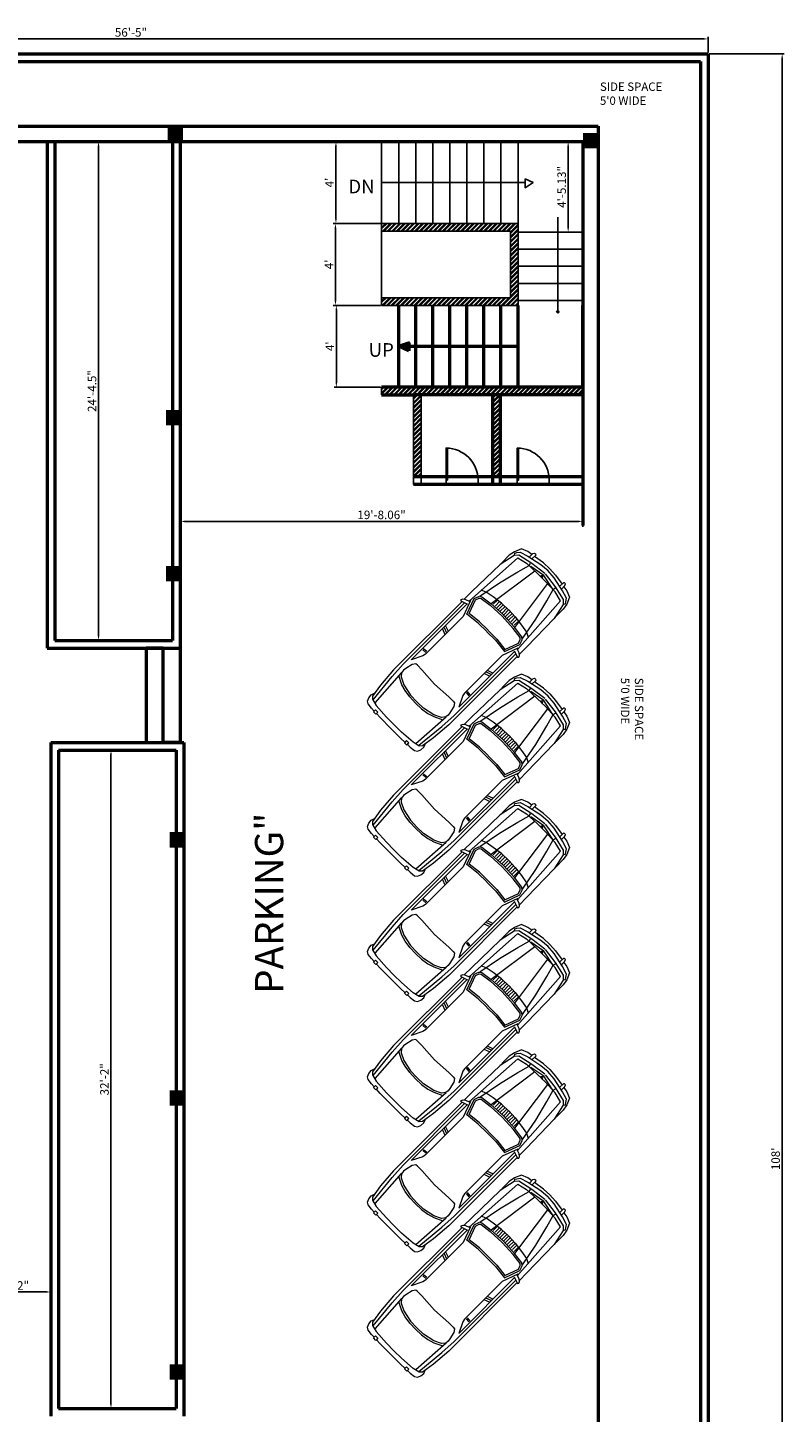
# Model space of a CAD drawing. Units: inches. Extents: x -2733 to 3435, y -338 to 1843.
# Tile 4 of 7: x -2146 to -1702, y 764 to 1575. Entities that reach past the tile are written whole.
import ezdxf

# ---------------------------------------------------------------- set-up
doc = ezdxf.new("R2010")
doc.units = ezdxf.units.IN
doc.header["$PDMODE"] = 34
for name, color, linetype, lineweight in [('A-ANNO-DIMS', 2, 'Continuous', 18), ('A-ANNO-TEXT', 7, 'Continuous', 18), ('A-AREA-IDEN', 3, 'Continuous', 18), ('A-COLS', 1, 'Continuous', 35), ('A-DOOR', 1, 'Continuous', 25), ('A-FLOR-STRS', 4, 'Continuous', 25), ('A-WALL', 7, 'Continuous', 50), ('A-WALL-PATT', 8, 'Continuous', 13), ('C-PRKG', 8, 'Continuous', 18)]:
    doc.layers.add(name, color=color, linetype=linetype, lineweight=lineweight)
doc.styles.get("Standard").update_dxf_attribs({"font": 'arial.ttf'})
doc.styles.add('YQ_DIM', font='SUPEROS.SHX', dxfattribs={"width": 0.8, "bigfont": 'HZDX.SHX'})
doc.dimstyles.new('ISO-25', dxfattribs={"dimtxt": 5, "dimasz": 2.5, "dimexe": 1.25, "dimexo": 0.625, "dimtad": 1, "dimlunit": 3, "dimtxsty": 'Standard', "dimcen": 2.5, "dimadec": 0, "dimazin": 0, "dimtfac": 1, "dimtmove": 0, "dimatfit": 3, "dimfxl": 1, "dimarcsym": 0})

# ---------------------------------------------------------------- blocks, each defined once
blk = doc.blocks.new('A$C49703025')
for p, q in [((-0.089, 0.573), (-0.077, 0.686)), ((-0.077, 0.686), (-0.044, 0.735)), ((-0.044, 0.735), (0.024, 0.765)), ((0.057, 0.691), (0.02, 0.543)), ((0.024, 0.765), (0.105, 0.775)), ((0.881, 0.661), (0.04, 0.607)), ((0.105, 0.735), (0.057, 0.691)), ((0.061, 0.671), (0.683, 0.735)), ((0.388, 0.78), (0.105, 0.735)), ((0.105, 0.775), (0.174, 0.75)), ((0.804, 0.813), (0.388, 0.78)), ((0.683, 0.735), (1.027, 0.755)), ((0.707, 0.469), (0.792, 0.652)), ((0.808, 0.597), (0.732, 0.444)), ((2.822, 0.813), (0.804, 0.813)), ((0.877, 0.652), (0.808, 0.597)), ((0.942, 0.661), (0.877, 0.652)), ((1.002, 0.652), (0.942, 0.661)), ((1.152, 0.617), (1.002, 0.652)), ((1.027, 0.755), (2.841, 0.755)), ((1.217, 0.573), (1.152, 0.617)), ((1.443, 0.586), (1.212, 0.702)), ((1.212, 0.702), (2.85, 0.702)), ((1.507, 0.575), (1.443, 0.586)), ((1.538, 0.592), (1.529, 0.68)), ((1.566, 0.592), (1.557, 0.68)), ((2.125, 0.696), (2.083, 0.58)), ((2.174, 0.695), (2.132, 0.579)), ((2.219, 0.697), (2.178, 0.581)), ((2.958, 0.702), (2.618, 0.575)), ((2.707, 0.554), (3.041, 0.676)), ((2.747, 0.529), (3.041, 0.637)), ((2.816, 0.829), (2.838, 0.849)), ((2.864, 0.684), (2.816, 0.829)), ((2.838, 0.849), (2.874, 0.835)), ((2.874, 0.835), (2.905, 0.791)), ((3.1, 0.813), (2.89, 0.813)), ((2.905, 0.791), (2.932, 0.714)), ((2.932, 0.714), (4.286, 0.632)), ((3.041, 0.676), (3.144, 0.639)), ((3.041, 0.637), (3.122, 0.608)), ((3.929, 0.795), (3.1, 0.813)), ((3.122, 0.608), (3.148, 0.576)), ((3.144, 0.639), (3.183, 0.591)), ((3.163, 0.627), (3.648, 0.536)), ((3.183, 0.591), (3.217, 0.343)), ((3.317, 0.591), (3.271, 0.695)), ((3.35, 0.417), (3.317, 0.591)), ((4.269, 0.722), (3.929, 0.795)), ((3.993, 0.795), (3.965, 0.787)), ((4.2, 0.795), (3.993, 0.795)), ((4.328, 0.77), (4.2, 0.795)), ((4.343, 0.656), (4.269, 0.722)), ((4.279, 0.724), (4.312, 0.747)), ((4.286, 0.632), (4.337, 0.422)), ((4.312, 0.747), (4.35, 0.724)), ((4.472, 0.711), (4.328, 0.77)), ((4.412, 0.343), (4.343, 0.656)), ((4.35, 0.724), (4.407, 0.681)), ((4.407, 0.681), (4.461, 0.513)), ((4.525, 0.578), (4.472, 0.711)), ((-0.113, 0.489), (-0.053, 0.489)), ((-0.113, 0.42), (-0.113, 0.489)), ((-0.053, 0.42), (-0.113, 0.42)), ((-0.101, 0.306), (-0.096, 0.42)), ((-0.101, 0), (-0.101, 0.306)), ((-0.093, 0.489), (-0.089, 0.573)), ((-0.053, 0.489), (-0.053, 0.42)), ((0.02, 0.543), (0, 0.222)), ((0.643, 0.173), (0.667, 0.336)), ((0.667, 0.336), (0.707, 0.469)), ((0.732, 0.444), (0.679, 0.193)), ((1.196, 0), (1.221, 0.4)), ((1.221, 0.528), (1.217, 0.573)), ((1.221, 0.4), (1.221, 0.528)), ((2.618, 0.575), (1.507, 0.575)), ((2.741, 0.254), (2.707, 0.554)), ((2.778, 0.256), (2.747, 0.529)), ((3.148, 0.576), (3.18, 0.34)), ((3.18, 0.34), (3.198, 0)), ((3.217, 0.343), (3.235, 0.002)), ((3.22, 0.35), (4.35, 0.19)), ((3.241, 0.309), (3.365, 0.309)), ((3.38, 0.202), (3.35, 0.417)), ((3.648, 0.536), (4.083, 0.427)), ((4.083, 0.427), (4.344, 0.354)), ((4.337, 0.422), (4.348, 0.111)), ((4.344, 0.354), (4.395, 0.364)), ((4.415, -0.011), (4.354, 0.313)), ((4.395, 0.364), (4.404, 0.379)), ((4.456, 0.006), (4.412, 0.343)), ((4.461, 0.513), (4.529, 0.197)), ((4.473, 0.474), (4.574, 0.474)), ((4.592, 0.408), (4.49, 0.408)), ((4.542, 0.474), (4.525, 0.578)), ((4.59, 0.18), (4.553, 0.408)), ((4.574, 0.474), (4.606, 0.455)), ((4.609, 0.429), (4.592, 0.408)), ((4.606, 0.455), (4.609, 0.429)), ((-0.101, 0), (-0.101, -0.306)), ((0, 0.222), (0, 0)), ((0, -0.222), (0, 0)), ((0.635, 0), (0.643, 0.173)), ((0.635, 0), (0.643, -0.173)), ((0.679, 0.193), (0.671, 0)), ((0.679, -0.193), (0.671, 0)), ((1.196, 0), (1.221, -0.4)), ((2.744, 0.002), (2.741, 0.254)), ((2.781, 0.003), (2.778, 0.256)), ((3.241, 0.257), (3.373, 0.257)), ((3.241, 0.206), (3.382, 0.206)), ((3.241, 0.154), (3.382, 0.154)), ((3.241, 0.103), (3.382, 0.103)), ((3.241, 0.051), (3.382, 0.051)), ((3.241, 0), (3.382, 0)), ((3.386, 0.002), (3.38, 0.202)), ((4.348, 0.111), (4.348, -0.004)), ((4.348, -0.111), (4.348, 0.004)), ((4.363, 0.028), (4.359, 0.005)), ((4.359, 0.005), (4.363, -0.023)), ((4.386, 0.005), (4.363, 0.028)), ((4.529, 0.197), (4.546, -0.002)), ((4.529, -0.197), (4.546, 0.002)), ((4.599, 0), (4.59, 0.18)), ((4.599, 0), (4.59, -0.18)), ((0.02, -0.543), (0, -0.222)), ((0.643, -0.173), (0.667, -0.336)), ((0.732, -0.444), (0.679, -0.193)), ((2.741, -0.254), (2.707, -0.554)), ((2.744, -0.002), (2.741, -0.254)), ((2.778, -0.256), (2.747, -0.529)), ((2.781, -0.003), (2.778, -0.256)), ((3.18, -0.34), (3.198, 0)), ((3.217, -0.343), (3.235, -0.002)), ((3.22, -0.35), (4.35, -0.19)), ((3.241, -0.051), (3.382, -0.051)), ((3.241, -0.103), (3.382, -0.103)), ((3.241, -0.154), (3.382, -0.154)), ((3.241, -0.206), (3.382, -0.206)), ((3.241, -0.257), (3.373, -0.257)), ((3.38, -0.202), (3.35, -0.417)), ((3.386, -0.002), (3.38, -0.202)), ((4.337, -0.422), (4.348, -0.111)), ((4.344, -0.347), (4.415, -0.011)), ((4.401, 0), (4.354, 0)), ((4.363, -0.023), (4.382, -0.011)), ((4.456, -0.006), (4.412, -0.343)), ((4.461, -0.513), (4.529, -0.197)), ((4.59, -0.18), (4.553, -0.408)), ((-0.053, -0.42), (-0.113, -0.42)), ((-0.113, -0.42), (-0.113, -0.489)), ((-0.113, -0.489), (-0.053, -0.489)), ((-0.101, -0.306), (-0.096, -0.42)), ((-0.093, -0.489), (-0.089, -0.573)), ((-0.089, -0.573), (-0.077, -0.686)), ((-0.053, -0.489), (-0.053, -0.42)), ((0.057, -0.691), (0.02, -0.543)), ((0.667, -0.336), (0.707, -0.469)), ((0.707, -0.469), (0.792, -0.652)), ((0.808, -0.597), (0.732, -0.444)), ((1.217, -0.573), (1.152, -0.617)), ((1.221, -0.528), (1.217, -0.573)), ((1.221, -0.4), (1.221, -0.528)), ((1.507, -0.575), (1.443, -0.586)), ((2.618, -0.575), (1.507, -0.575)), ((2.958, -0.702), (2.618, -0.575)), ((2.707, -0.554), (3.041, -0.676)), ((2.747, -0.529), (3.041, -0.637)), ((3.122, -0.608), (3.148, -0.576)), ((3.148, -0.576), (3.18, -0.34)), ((3.163, -0.627), (3.648, -0.536)), ((3.183, -0.591), (3.217, -0.343)), ((3.241, -0.309), (3.365, -0.309)), ((3.35, -0.417), (3.317, -0.591)), ((3.648, -0.536), (4.083, -0.427)), ((4.083, -0.427), (4.344, -0.354)), ((4.286, -0.632), (4.337, -0.422)), ((4.412, -0.343), (4.343, -0.656)), ((4.344, -0.354), (4.395, -0.364)), ((4.395, -0.364), (4.404, -0.379)), ((4.407, -0.681), (4.461, -0.513)), ((4.525, -0.578), (4.472, -0.711)), ((4.473, -0.474), (4.574, -0.474)), ((4.592, -0.408), (4.49, -0.408)), ((4.542, -0.474), (4.525, -0.578)), ((4.574, -0.474), (4.606, -0.455)), ((4.609, -0.429), (4.592, -0.408)), ((4.606, -0.455), (4.609, -0.429)), ((-0.077, -0.686), (-0.044, -0.735)), ((-0.044, -0.735), (0.024, -0.765)), ((0.024, -0.765), (0.105, -0.775)), ((0.881, -0.661), (0.04, -0.607)), ((0.105, -0.735), (0.057, -0.691)), ((0.061, -0.671), (0.683, -0.735)), ((0.388, -0.78), (0.105, -0.735)), ((0.105, -0.775), (0.174, -0.75)), ((0.804, -0.813), (0.388, -0.78)), ((0.683, -0.735), (1.027, -0.755)), ((2.822, -0.813), (0.804, -0.813)), ((0.877, -0.652), (0.808, -0.597)), ((0.942, -0.661), (0.877, -0.652)), ((1.002, -0.652), (0.942, -0.661)), ((1.152, -0.617), (1.002, -0.652)), ((1.027, -0.755), (2.841, -0.755)), ((1.443, -0.586), (1.212, -0.702)), ((1.212, -0.702), (2.85, -0.702)), ((1.538, -0.592), (1.529, -0.68)), ((1.566, -0.592), (1.557, -0.68)), ((2.125, -0.696), (2.083, -0.58)), ((2.174, -0.695), (2.132, -0.579)), ((2.219, -0.697), (2.178, -0.581)), ((2.864, -0.684), (2.816, -0.829)), ((2.816, -0.829), (2.838, -0.849)), ((2.838, -0.849), (2.874, -0.835)), ((2.874, -0.835), (2.905, -0.791)), ((3.1, -0.813), (2.89, -0.813)), ((2.905, -0.791), (2.932, -0.714)), ((2.932, -0.714), (4.286, -0.632)), ((3.041, -0.637), (3.122, -0.608)), ((3.041, -0.676), (3.144, -0.639)), ((3.929, -0.795), (3.1, -0.813)), ((3.144, -0.639), (3.183, -0.591)), ((3.317, -0.591), (3.271, -0.695)), ((4.269, -0.722), (3.929, -0.795)), ((3.993, -0.795), (3.965, -0.787)), ((4.2, -0.795), (3.993, -0.795)), ((4.328, -0.77), (4.2, -0.795)), ((4.343, -0.656), (4.269, -0.722)), ((4.279, -0.724), (4.312, -0.747)), ((4.312, -0.747), (4.35, -0.724)), ((4.472, -0.711), (4.328, -0.77)), ((4.35, -0.724), (4.407, -0.681))]:
    blk.add_line(p, q)
blk = doc.blocks.new('*D6')
at = {"layer": 'A-ANNO-DIMS', "color": 0, "lineweight": -2, "transparency": 16777216}
for p, q in [((-1745.94, 1560.13), (-1701.93, 1560.13)), ((-1703.18, 1557.63), (-1703.18, 266.63)), ((-1745.94, 264.13), (-1701.93, 264.13))]:
    blk.add_line(p, q, dxfattribs=at)
at = {"layer": 'A-ANNO-DIMS', "color": 0, "lineweight": 20, "transparency": 16777216}
for points in [[(-1703.6, 1557.63), (-1702.76, 1557.63), (-1703.18, 1560.13)], [(-1703.6, 266.63), (-1702.76, 266.63), (-1703.18, 264.13)]]:
    blk.add_solid(points, dxfattribs=at)
at = {"layer": 'Defpoints', "color": 0, "lineweight": 20, "transparency": 16777216}
for p in [(-1746.57, 1560.13), (-1746.57, 264.13), (-1703.18, 264.13)]:
    blk.add_point(p, dxfattribs=at)
at = {"layer": 'A-ANNO-DIMS', "color": 0, "transparency": 16777216, "insert": (-1706.36, 912.13), "char_height": 5, "attachment_point": 5, "rotation": 90}
blk.add_mtext("108'", dxfattribs=at)
blk = doc.blocks.new('*D8')
at = {"layer": 'A-ANNO-DIMS', "color": 0, "lineweight": -2, "transparency": 16777216}
for p, q in [((-2093.63, 1151.77), (-2098.01, 1151.77)), ((-2096.76, 1149.27), (-2096.76, 768.27)), ((-2093.63, 765.77), (-2098.01, 765.77))]:
    blk.add_line(p, q, dxfattribs=at)
at = {"layer": 'A-ANNO-DIMS', "color": 0, "lineweight": 20, "transparency": 16777216}
for points in [[(-2097.18, 1149.27), (-2096.34, 1149.27), (-2096.76, 1151.77)], [(-2097.18, 768.27), (-2096.34, 768.27), (-2096.76, 765.77)]]:
    blk.add_solid(points, dxfattribs=at)
at = {"layer": 'Defpoints', "color": 0, "lineweight": 20, "transparency": 16777216}
for p in [(-2093.01, 1151.77), (-2096.76, 765.77), (-2093.01, 765.77)]:
    blk.add_point(p, dxfattribs=at)
at = {"layer": 'A-ANNO-DIMS', "color": 0, "transparency": 16777216, "insert": (-2099.94, 958.77), "char_height": 5, "attachment_point": 5, "rotation": 90}
blk.add_mtext('32\'-2"', dxfattribs=at)
blk = doc.blocks.new('*D9')
at = {"layer": 'A-ANNO-DIMS', "color": 0, "lineweight": -2, "transparency": 16777216}
for p, q in [((-2182.13, 829.34), (-2182.13, 835.34)), ((-2179.63, 834.09), (-2134.51, 834.09)), ((-2132.01, 829.34), (-2132.01, 835.34))]:
    blk.add_line(p, q, dxfattribs=at)
at = {"layer": 'A-ANNO-DIMS', "color": 0, "lineweight": 20, "transparency": 16777216}
for points in [[(-2179.63, 834.5), (-2179.63, 833.67), (-2182.13, 834.09)], [(-2134.51, 834.5), (-2134.51, 833.67), (-2132.01, 834.09)]]:
    blk.add_solid(points, dxfattribs=at)
at = {"layer": 'Defpoints', "color": 0, "lineweight": 20, "transparency": 16777216}
for p in [(-2182.13, 828.71), (-2132.01, 834.09), (-2132.01, 828.71)]:
    blk.add_point(p, dxfattribs=at)
at = {"layer": 'A-ANNO-DIMS', "color": 0, "transparency": 16777216, "insert": (-2157.07, 837.22), "char_height": 5, "attachment_point": 5}
blk.add_mtext('4\'-2.12"', dxfattribs=at)
blk = doc.blocks.new('*D12')
at = {"layer": 'A-ANNO-DIMS', "color": 0, "lineweight": -2, "transparency": 16777216}
for p, q in [((-2094.22, 1508.58), (-2105.31, 1508.58)), ((-2104.06, 1506.08), (-2104.06, 1218.58)), ((-2100.09, 1216.08), (-2105.31, 1216.08))]:
    blk.add_line(p, q, dxfattribs=at)
at = {"layer": 'A-ANNO-DIMS', "color": 0, "lineweight": 20, "transparency": 16777216}
for points in [[(-2104.47, 1506.08), (-2103.64, 1506.08), (-2104.06, 1508.58)], [(-2104.47, 1218.58), (-2103.64, 1218.58), (-2104.06, 1216.08)]]:
    blk.add_solid(points, dxfattribs=at)
at = {"layer": 'Defpoints', "color": 0, "lineweight": 20, "transparency": 16777216}
for p in [(-2093.59, 1508.58), (-2104.06, 1216.08), (-2099.46, 1216.08)]:
    blk.add_point(p, dxfattribs=at)
at = {"layer": 'A-ANNO-DIMS', "color": 0, "transparency": 16777216, "insert": (-2107.23, 1362.33), "char_height": 5, "attachment_point": 5, "rotation": 90}
blk.add_mtext('24\'-4.5"', dxfattribs=at)
blk = doc.blocks.new('*D13')
at = {"layer": 'A-ANNO-DIMS', "color": 0, "lineweight": -2, "transparency": 16777216}
for p, q in [((-2423.57, 1560.75), (-2423.57, 1570.04)), ((-2421.07, 1568.79), (-1749.07, 1568.79)), ((-1746.57, 1560.75), (-1746.57, 1570.04))]:
    blk.add_line(p, q, dxfattribs=at)
at = {"layer": 'A-ANNO-DIMS', "color": 0, "lineweight": 20, "transparency": 16777216}
for points in [[(-2421.07, 1569.21), (-2421.07, 1568.38), (-2423.57, 1568.79)], [(-1749.07, 1569.21), (-1749.07, 1568.38), (-1746.57, 1568.79)]]:
    blk.add_solid(points, dxfattribs=at)
at = {"layer": 'Defpoints', "color": 0, "lineweight": 20, "transparency": 16777216}
for p in [(-1746.57, 1568.79), (-2423.57, 1560.13), (-1746.57, 1560.13)]:
    blk.add_point(p, dxfattribs=at)
at = {"layer": 'A-ANNO-DIMS', "color": 0, "transparency": 16777216, "insert": (-2085.07, 1571.97), "char_height": 5, "attachment_point": 5}
blk.add_mtext('56\'-5"', dxfattribs=at)
blk = doc.blocks.new('*D14')
at = {"layer": 'A-ANNO-DIMS', "color": 0, "lineweight": -2, "transparency": 16777216}
for p, q in [((-1830.95, 1508.58), (-1827.42, 1508.58)), ((-1828.67, 1506.08), (-1828.67, 1457.96)), ((-1828.59, 1455.46), (-1827.42, 1455.46))]:
    blk.add_line(p, q, dxfattribs=at)
at = {"layer": 'A-ANNO-DIMS', "color": 0, "lineweight": 20, "transparency": 16777216}
for points in [[(-1829.09, 1506.08), (-1828.26, 1506.08), (-1828.67, 1508.58)], [(-1829.09, 1457.96), (-1828.26, 1457.96), (-1828.67, 1455.46)]]:
    blk.add_solid(points, dxfattribs=at)
at = {"layer": 'Defpoints', "color": 0, "lineweight": 20, "transparency": 16777216}
for p in [(-1831.58, 1508.58), (-1829.22, 1455.46), (-1828.67, 1455.46)]:
    blk.add_point(p, dxfattribs=at)
at = {"layer": 'A-ANNO-DIMS', "color": 0, "transparency": 16777216, "insert": (-1831.85, 1482.02), "char_height": 5, "attachment_point": 5, "rotation": 90}
blk.add_mtext('4\'-5.13"', dxfattribs=at)
blk = doc.blocks.new('*D15')
at = {"layer": 'A-ANNO-DIMS', "color": 0, "lineweight": -2, "transparency": 16777216}
for p, q in [((-1963.16, 1508.58), (-1966.11, 1508.58)), ((-1964.86, 1506.08), (-1964.86, 1463.08)), ((-1938.69, 1460.58), (-1966.11, 1460.58))]:
    blk.add_line(p, q, dxfattribs=at)
at = {"layer": 'A-ANNO-DIMS', "color": 0, "lineweight": 20, "transparency": 16777216}
for points in [[(-1965.27, 1506.08), (-1964.44, 1506.08), (-1964.86, 1508.58)], [(-1965.27, 1463.08), (-1964.44, 1463.08), (-1964.86, 1460.58)]]:
    blk.add_solid(points, dxfattribs=at)
at = {"layer": 'Defpoints', "color": 0, "lineweight": 20, "transparency": 16777216}
for p in [(-1962.53, 1508.58), (-1964.86, 1460.58), (-1938.07, 1460.58)]:
    blk.add_point(p, dxfattribs=at)
at = {"layer": 'A-ANNO-DIMS', "color": 0, "transparency": 16777216, "insert": (-1967.98, 1484.58), "char_height": 5, "attachment_point": 5, "rotation": 90}
blk.add_mtext("4'", dxfattribs=at)
blk = doc.blocks.new('*D16')
at = {"layer": 'A-ANNO-DIMS', "color": 0, "lineweight": -2, "transparency": 16777216}
for p, q in [((-1938.69, 1460.58), (-1966.4, 1460.58)), ((-1965.15, 1458.08), (-1965.15, 1415.08)), ((-1938.69, 1412.58), (-1966.4, 1412.58))]:
    blk.add_line(p, q, dxfattribs=at)
at = {"layer": 'A-ANNO-DIMS', "color": 0, "lineweight": 20, "transparency": 16777216}
for points in [[(-1965.56, 1458.08), (-1964.73, 1458.08), (-1965.15, 1460.58)], [(-1965.56, 1415.08), (-1964.73, 1415.08), (-1965.15, 1412.58)]]:
    blk.add_solid(points, dxfattribs=at)
at = {"layer": 'Defpoints', "color": 0, "lineweight": 20, "transparency": 16777216}
for p in [(-1938.07, 1460.58), (-1965.15, 1412.58), (-1938.07, 1412.58)]:
    blk.add_point(p, dxfattribs=at)
at = {"layer": 'A-ANNO-DIMS', "color": 0, "transparency": 16777216, "insert": (-1968.27, 1436.58), "char_height": 5, "attachment_point": 5, "rotation": 90}
blk.add_mtext("4'", dxfattribs=at)
blk = doc.blocks.new('*D17')
at = {"layer": 'A-ANNO-DIMS', "color": 0, "lineweight": -2, "transparency": 16777216}
for p, q in [((-1938.69, 1412.58), (-1965.87, 1412.58)), ((-1964.62, 1410.08), (-1964.62, 1367.08)), ((-1938.69, 1364.58), (-1965.87, 1364.58))]:
    blk.add_line(p, q, dxfattribs=at)
at = {"layer": 'A-ANNO-DIMS', "color": 0, "lineweight": 20, "transparency": 16777216}
for points in [[(-1965.04, 1410.08), (-1964.21, 1410.08), (-1964.62, 1412.58)], [(-1965.04, 1367.08), (-1964.21, 1367.08), (-1964.62, 1364.58)]]:
    blk.add_solid(points, dxfattribs=at)
at = {"layer": 'Defpoints', "color": 0, "lineweight": 20, "transparency": 16777216}
for p in [(-1938.07, 1412.58), (-1964.62, 1364.58), (-1938.07, 1364.58)]:
    blk.add_point(p, dxfattribs=at)
at = {"layer": 'A-ANNO-DIMS', "color": 0, "transparency": 16777216, "insert": (-1967.75, 1388.58), "char_height": 5, "attachment_point": 5, "rotation": 90}
blk.add_mtext("4'", dxfattribs=at)
blk = doc.blocks.new('*D18')
at = {"layer": 'A-ANNO-DIMS', "color": 0, "lineweight": -2, "transparency": 16777216}
for p, q in [((-2056.13, 1282.79), (-2056.13, 1287.15)), ((-2053.63, 1285.9), (-1822.57, 1285.9)), ((-1820.07, 1282.79), (-1820.07, 1287.15))]:
    blk.add_line(p, q, dxfattribs=at)
at = {"layer": 'A-ANNO-DIMS', "color": 0, "lineweight": 20, "transparency": 16777216}
for points in [[(-2053.63, 1286.32), (-2053.63, 1285.49), (-2056.13, 1285.9)], [(-1822.57, 1286.32), (-1822.57, 1285.49), (-1820.07, 1285.9)]]:
    blk.add_solid(points, dxfattribs=at)
at = {"layer": 'Defpoints', "color": 0, "lineweight": 20, "transparency": 16777216}
for p in [(-1820.07, 1285.9), (-2056.13, 1282.16), (-1820.07, 1282.16)]:
    blk.add_point(p, dxfattribs=at)
at = {"layer": 'A-ANNO-DIMS', "color": 0, "transparency": 16777216, "insert": (-1938.1, 1289.08), "char_height": 5, "width": 26.4154, "attachment_point": 5}
blk.add_mtext('19\'-8.06"', dxfattribs=at)
blk = doc.blocks.new('*U21')
for p, q in [((0, 0), (0, -6)), ((40, 0), (40, -6))]:
    blk.add_line(p, q)
blk.add_lwpolyline([(0, 0), (0, 40), (1.75, 40), (1.75, 0)], close=True)
blk.add_arc((0, 0), 40, 0, 90)

msp = doc.modelspace()

# ---------------------------------------------------------------- hatches: boundary and pattern name
at = {"layer": 'A-COLS'}
h = msp.add_hatch(color=256, dxfattribs=at)
h.dxf.hatch_style = 1
h.paths.add_polyline_path([(-2054.447, 1517.797), (-2063.447, 1517.797), (-2063.447, 1508.797), (-2054.447, 1508.797)])
h = msp.add_hatch(color=256, dxfattribs=at)
h.dxf.hatch_style = 1
h.paths.add_polyline_path([(-1811.069, 1513.681), (-1820.069, 1513.681), (-1820.069, 1504.681), (-1811.069, 1504.681)])
h = msp.add_hatch(color=256, dxfattribs=at)
h.dxf.hatch_style = 1
h.paths.add_polyline_path([(-2055.55, 1351.181), (-2064.55, 1351.181), (-2064.55, 1342.181), (-2055.55, 1342.181)])
h = msp.add_hatch(color=256, dxfattribs=at)
h.dxf.hatch_style = 1
h.paths.add_polyline_path([(-2055.55, 1259.681), (-2064.55, 1259.681), (-2064.55, 1250.681), (-2055.55, 1250.681)])
h = msp.add_hatch(color=256, dxfattribs=at)
h.dxf.hatch_style = 1
h.paths.add_polyline_path([(-2053.43, 1103.681), (-2062.43, 1103.681), (-2062.43, 1094.681), (-2053.43, 1094.681)])
h = msp.add_hatch(color=256, dxfattribs=at)
h.dxf.hatch_style = 1
h.paths.add_polyline_path([(-2053.43, 952.373), (-2062.43, 952.373), (-2062.43, 943.373), (-2053.43, 943.373)])
h = msp.add_hatch(color=256, dxfattribs=at)
h.dxf.hatch_style = 1
h.paths.add_polyline_path([(-2053.43, 791.681), (-2062.43, 791.681), (-2062.43, 782.681), (-2053.43, 782.681)])
at = {"layer": 'A-WALL-PATT'}
h = msp.add_hatch(dxfattribs=at)
h.set_pattern_fill('ANSI32', color=256, scale=0.2)
h.set_pattern_definition([(45, (-2862.9097, 0), (-1.3470384, 1.3470384), []), (45, (-2862.0116, 0), (-1.3470384, 1.3470384), [])])
h.paths.add_polyline_path([(-1858.069, 1460.58), (-1938.069, 1460.58), (-1938.069, 1456.08), (-1862.569, 1456.08), (-1862.569, 1417.08), (-1938.069, 1417.08), (-1938.069, 1412.58), (-1858.069, 1412.58)])
h.paths.add_polyline_path([(-1820.069, 1364.58), (-1926.069, 1364.58), (-1938.069, 1364.58), (-1938.069, 1360.08), (-1919.411, 1360.08), (-1820.069, 1360.08)])
h.paths.add_polyline_path([(-1868.411, 1360.08), (-1872.911, 1360.08), (-1872.911, 1312.08), (-1868.411, 1312.08)])
h.paths.add_polyline_path([(-1914.911, 1360.08), (-1919.411, 1360.08), (-1919.411, 1312.08), (-1914.911, 1312.08)])

# ---------------------------------------------------------------- linework, layer by layer
at = {"layer": 'A-FLOR-STRS'}
for p, q in [((-1938.069, 1460.58), (-1938.069, 1508.58)), ((-1938.069, 1508.58), (-1938.069, 1460.58)), ((-1928.069, 1508.58), (-1928.069, 1460.58)), ((-1918.069, 1508.58), (-1918.069, 1460.58)), ((-1908.069, 1508.58), (-1908.069, 1460.58)), ((-1898.069, 1508.58), (-1898.069, 1460.58)), ((-1888.069, 1508.58), (-1888.069, 1460.58)), ((-1878.069, 1508.58), (-1878.069, 1460.58)), ((-1868.069, 1508.58), (-1868.069, 1460.58)), ((-1858.069, 1508.58), (-1858.069, 1460.58)), ((-1938.069, 1484.58), (-1853.976, 1484.58)), ((-1834.724, 1464.214), (-1834.724, 1409.038)), ((-1858.069, 1455.455), (-1820.069, 1455.455)), ((-1858.069, 1445.455), (-1820.069, 1445.455)), ((-1858.069, 1435.455), (-1820.069, 1435.455)), ((-1858.069, 1425.455), (-1820.069, 1425.455)), ((-1858.069, 1415.455), (-1820.069, 1415.455)), ((-1834.724, 1409.048), (-1835.743, 1409.048)), ((-1835.743, 1409.048), (-1834.724, 1407.913)), ((-1834.724, 1410.594), (-1834.724, 1409.048)), ((-1834.724, 1409.038), (-1833.881, 1409.038)), ((-1833.881, 1409.038), (-1834.724, 1407.913)), ((-1938.069, 1364.58), (-1938.069, 1360.08)), ((-1919.411, 1307.58), (-1919.411, 1360.08)), ((-1914.911, 1307.58), (-1914.911, 1360.08))]:
    msp.add_line(p, q, dxfattribs=at)
for points in [[(-1853.976, 1486.823), (-1853.976, 1481.574), (-1849.224, 1484.58)], [(-1938.069, 1412.58), (-1858.069, 1412.58), (-1858.069, 1460.58), (-1938.069, 1460.58)]]:
    msp.add_lwpolyline(points, close=True, dxfattribs=at)
msp.add_lwpolyline([(-1938.069, 1417.08), (-1862.569, 1417.08), (-1862.569, 1456.08), (-1938.069, 1456.08)], dxfattribs=at)
at = {"layer": 'A-WALL'}
for p, q in [((-2423.568, 1560.127), (-1746.569, 1560.127)), ((-1746.569, 1560.127), (-1746.569, 264.127)), ((-2419.298, 1555.627), (-1751.069, 1555.627)), ((-1751.069, 1555.627), (-1751.069, 266.673)), ((-2361.21, 1517.58), (-1811.069, 1517.58)), ((-2340.407, 1517.58), (-1811.069, 1517.58)), ((-1811.069, 1517.58), (-1811.069, 503.08)), ((-1811.069, 1517.58), (-1811.069, 513.58)), ((-2352.669, 1508.58), (-1820.069, 1508.58)), ((-2348.399, 1508.58), (-1820.069, 1508.58)), ((-2134.126, 1508.58), (-2134.126, 1211.58)), ((-2129.626, 1508.58), (-2129.626, 1216.08)), ((-2060.626, 1508.58), (-2060.626, 1216.08)), ((-2056.126, 1508.58), (-2056.126, 1211.58)), ((-1820.069, 1508.58), (-1820.069, 1283.58)), ((-1928.069, 1364.58), (-1928.069, 1412.58)), ((-1918.069, 1364.58), (-1918.069, 1412.58)), ((-1908.069, 1364.58), (-1908.069, 1412.58)), ((-1898.069, 1364.58), (-1898.069, 1412.58)), ((-1888.069, 1364.58), (-1888.069, 1412.58)), ((-1878.069, 1364.58), (-1878.069, 1412.58)), ((-1868.069, 1364.58), (-1868.069, 1412.58)), ((-1858.069, 1364.58), (-1858.069, 1412.58)), ((-1820.069, 1364.58), (-1820.069, 1412.58)), ((-1928.069, 1388.58), (-1858.069, 1388.58)), ((-1926.069, 1364.58), (-1938.069, 1364.58)), ((-1820.069, 1364.58), (-1926.069, 1364.58)), ((-1938.069, 1360.08), (-1919.411, 1360.08)), ((-1820.069, 1360.08), (-1919.411, 1360.08)), ((-1872.911, 1307.58), (-1872.911, 1360.08)), ((-1868.411, 1307.58), (-1868.411, 1360.08)), ((-1820.069, 1312.08), (-1919.411, 1312.08)), ((-1820.069, 1307.58), (-1919.411, 1307.58)), ((-2134.126, 1211.58), (-2056.126, 1211.58)), ((-2129.626, 1216.08), (-2060.626, 1216.08)), ((-2066.126, 1211.58), (-2076.126, 1211.58)), ((-2076.126, 1211.58), (-2076.126, 1156.269)), ((-2066.126, 1156.269), (-2066.126, 1211.58)), ((-2056.126, 1211.58), (-2056.126, 1156.269)), ((-2132.006, 1156.269), (-2054.006, 1156.269)), ((-2132.006, 1156.269), (-2132.006, 761.269)), ((-2056.126, 1156.269), (-2066.126, 1156.269)), ((-2054.006, 1156.269), (-2054.006, 761.269)), ((-2127.506, 1151.769), (-2127.506, 765.769)), ((-2127.506, 1151.769), (-2058.506, 1151.769)), ((-2058.506, 1151.769), (-2058.506, 765.769)), ((-2127.506, 765.769), (-2058.506, 765.769))]:
    msp.add_line(p, q, dxfattribs=at)
msp.add_lwpolyline([(-1922.125, 1385.99), (-1928.069, 1388.58), (-1922.125, 1390.5)], close=True, dxfattribs=at)

# ---------------------------------------------------------------- block references
at = {"layer": 'A-DOOR', "xscale": 0.468784832216934, "yscale": 0.468784832216934, "zscale": 0.468784832216934}
for p in [(-1900.275, 1310.099), (-1858.544, 1310.099)]:
    msp.add_blockref('*U21', p, dxfattribs=at)
at = {"layer": 'C-PRKG', "xscale": 28.10227870703558, "yscale": 28.10227870703558, "zscale": 28.10227870703558, "rotation": 45}
for p in [(-1930.847, 1166.749), (-1930.847, 1093.323), (-1930.847, 1019.897), (-1930.847, 946.472), (-1930.847, 873.046), (-1930.847, 799.62)]:
    msp.add_blockref('A$C49703025', p, dxfattribs=at)

# ---------------------------------------------------------------- texts
at = {"layer": 'A-ANNO-TEXT', "char_height": 8, "attachment_point": 1, "style": 'YQ_DIM'}
for s, insert in [('{\\fSitka Banner Semibold|b1|i0|c0|p2;DN}', (-1957.567, 1486.256)), ('{\\fSitka Banner Semibold|b1|i0|c0|p2;UP}', (-1945.689, 1390.421))]:
    msp.add_mtext_dynamic_manual_height_columns(s, width=3.68944, gutter_width=12.5, heights=[0], dxfattribs=dict(at, insert=insert))
at = {"layer": 'A-AREA-IDEN', "insert": (-1810.041, 1543.248), "char_height": 4.91305, "attachment_point": 1, "style": 'YQ_DIM'}
msp.add_mtext_dynamic_manual_height_columns("{\\f@Arial Unicode MS|b0|i0|c134|p34;SIDE SPACE\\P5'0 WIDE}", width=92.43125, gutter_width=24.565, heights=[0], dxfattribs=at)
at = {"layer": 'A-AREA-IDEN', "attachment_point": 1, "style": 'YQ_DIM'}
for s, width, gutter_width, insert, char_height, rotation in [("{\\f@Arial Unicode MS|b0|i0|c134|p34;SIDE SPACE\\P5'0 WIDE}", 92.43125, 24.565, (-1784.635, 1194.202), 4.91305, 270), ('{\\f@FZYaoTi|b0|i0|c134|p2;PARKING"}', 128.94034, 26.518, (-2012.336, 1008.891), 16.56819, 90)]:
    msp.add_mtext_dynamic_manual_height_columns(s, width=width, gutter_width=gutter_width, heights=[0], dxfattribs=dict(at, insert=insert, char_height=char_height, rotation=rotation))

# ---------------------------------------------------------------- dimensions: what is measured, and where the dimension line sits
at = {"layer": 'A-ANNO-DIMS'}
for base, p1, p2, picture, middle in [((-1746.569, 1568.792), (-2423.568, 1560.127), (-1746.569, 1560.127), '*D13', (-2085.069, 1571.97)), ((-1820.069, 1285.902), (-2056.126, 1282.163), (-1820.069, 1282.163), '*D18', (-1938.097, 1289.08)), ((-2132.006, 834.088), (-2182.126, 828.714), (-2132.006, 828.714), '*D9', (-2157.066, 837.223))]:
    dim = msp.add_linear_dim(base=base, p1=p1, p2=p2, dimstyle='ISO-25', override={"dimclrd": 0, "dimclre": 0, "dimclrt": 0}, dxfattribs=at)
    dim.commit()
    dim.dimension.update_dxf_attribs({"geometry": picture, "text_midpoint": middle})
for base, p1, p2, picture, middle in [((-1703.179, 264.127), (-1746.569, 1560.127), (-1746.569, 264.127), '*D6', (-1706.357, 912.127)), ((-2104.056, 1216.08), (-2093.594, 1508.58), (-2099.463, 1216.08), '*D12', (-2107.234, 1362.33)), ((-1964.855, 1460.58), (-1962.53, 1508.58), (-1938.069, 1460.58), '*D15', (-1967.98, 1484.58)), ((-1828.6746, 1455.45507), (-1831.57858, 1508.58014), (-1829.21909, 1455.45507), '*D14', (-1831.85417, 1482.01761)), ((-1965.146, 1412.58), (-1938.069, 1460.58), (-1938.069, 1412.58), '*D16', (-1968.271, 1436.58)), ((-1964.624, 1364.58), (-1938.069, 1412.58), (-1938.069, 1364.58), '*D17', (-1967.749, 1388.58)), ((-2096.76, 765.769), (-2093.006, 1151.769), (-2093.006, 765.769), '*D8', (-2099.94, 958.769))]:
    dim = msp.add_linear_dim(base=base, p1=p1, p2=p2, angle=90, dimstyle='ISO-25', override={"dimclrd": 0, "dimclre": 0, "dimclrt": 0}, dxfattribs=at)
    dim.commit()
    dim.dimension.update_dxf_attribs({"geometry": picture, "text_midpoint": middle})

doc.saveas('drawing.dxf')
